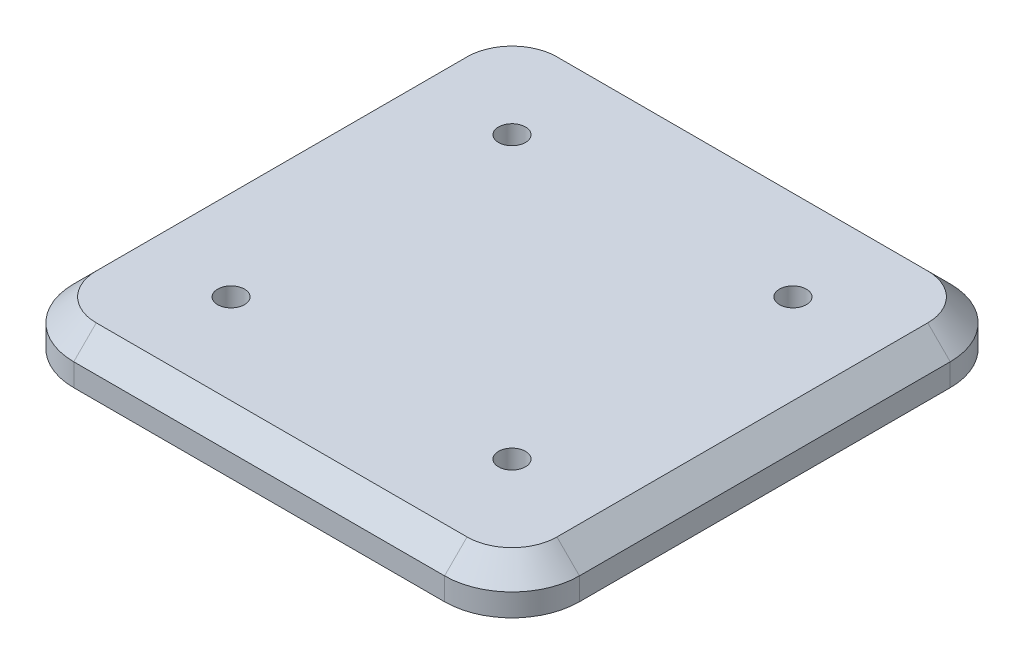
from build123d import *

# Parameters (mm, degrees)
BASE_PLATE_SKETCH_225X225_W        = 225
BASE_PLATE_SKETCH_225X225_H        = 225
BASE_PLATE_225X225X20_DEPTH        = 20
CORNER_FILLETS_R30_R               = 30
EDGE_CHAMFER_10X45_SIZE            = 10
DOWEL_HOLES_12_ON_125_LAYOUT_D     = 12
DOWEL_HOLES_12_ON_125_LAYOUT_DEPTH = 10
DOWEL_HOLES_12_ON_125_LAYOUT_TIP   = 3.605163714
DOWEL_HOLES_12_ON_175_LAYOUT_D     = 12
DOWEL_HOLES_12_ON_175_LAYOUT_DEPTH = 10
DOWEL_HOLES_12_ON_175_LAYOUT_TIP   = 3.605163714


with BuildPart() as part:
    # Base Plate Sketch 225x225 → Base Plate 225x225x20 (new body)
    with BuildSketch(Plane(origin=(0, 0, 0), x_dir=(1, 0, 0), z_dir=(0, 1, 0))):
        Rectangle(BASE_PLATE_SKETCH_225X225_W, BASE_PLATE_SKETCH_225X225_H)
    extrude(amount=BASE_PLATE_225X225X20_DEPTH)

    # Corner Fillets R30
    corner_fillets_r30_edges = [part.edges().sort_by_distance(p)[0] for p in [
        (112.5, 10, 112.5),
        (-112.5, 10, 112.5),
        (-112.5, 10, -112.5),
        (112.5, 10, -112.5),
    ]]
    fillet(corner_fillets_r30_edges, radius=CORNER_FILLETS_R30_R)

    # Edge Chamfer 10x45
    edge_chamfer_10x45_edges = [part.edges().sort_by_distance(p)[0] for p in [
        (-112.5, 20, 0),
        (0, 20, -112.5),
        (112.5, 20, 0),
        (0, 20, 112.5),
        (-103.713203436, 20, 103.713203436),
        (103.713203436, 20, 103.713203436),
        (103.713203436, 20, -103.713203436),
        (-103.713203436, 20, -103.713203436),
    ]]
    chamfer(edge_chamfer_10x45_edges, length=EDGE_CHAMFER_10X45_SIZE)

    # Dowel Holes Ø12 on 125 Layout
    with Locations(Plane(origin=(62.5, 20, 62.5), x_dir=(0, 0, 1), z_dir=(0, 1, 0))):
        with Locations((0, 0), (0, -125), (-125, -125), (-125, 0)):
            Hole(DOWEL_HOLES_12_ON_125_LAYOUT_D / 2, depth=DOWEL_HOLES_12_ON_125_LAYOUT_DEPTH)
            with Locations((0, 0, -(DOWEL_HOLES_12_ON_125_LAYOUT_DEPTH + DOWEL_HOLES_12_ON_125_LAYOUT_TIP / 2))):  # 118° drill point
                Cone(0, DOWEL_HOLES_12_ON_125_LAYOUT_D / 2, DOWEL_HOLES_12_ON_125_LAYOUT_TIP, mode=Mode.SUBTRACT)

    # Dowel Holes Ø12 on 175 Layout
    with Locations(Plane(origin=(-87.5, 0, 87.5), x_dir=(0, 0, -1), z_dir=(0, -1, 0))):
        with Locations((0, 0), (0, 175), (175, 175), (175, 0)):
            Hole(DOWEL_HOLES_12_ON_175_LAYOUT_D / 2, depth=DOWEL_HOLES_12_ON_175_LAYOUT_DEPTH)
            with Locations((0, 0, -(DOWEL_HOLES_12_ON_175_LAYOUT_DEPTH + DOWEL_HOLES_12_ON_175_LAYOUT_TIP / 2))):  # 118° drill point
                Cone(0, DOWEL_HOLES_12_ON_175_LAYOUT_D / 2, DOWEL_HOLES_12_ON_175_LAYOUT_TIP, mode=Mode.SUBTRACT)


solid = part.part
